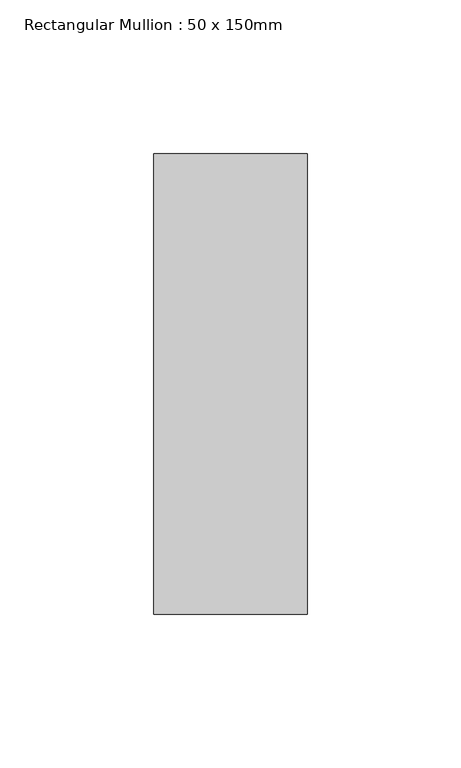
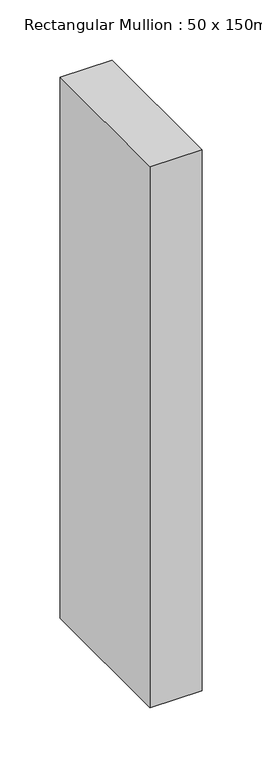
"""IFC4 building model written with IfcOpenShell, lengths in millimetres: member geometry, Rectangular Mullion : 50 x 150mm."""

from ifc_helpers import new_model, si_unit, frame, origin, place, context, project, spatial, polyline, outline, extrude, source, transform, mapped, element, save


def rectangular_mullion_50_x_150mm_b8dbbb25(model_context):
    return source(origin(), model_context, "Body", "SweptSolid", [
        extrude(outline(polyline([(25.0, 75.0), (25.0, -75.0), (-25.0, -75.0), (-25.0, 75.0), (25.0, 75.0)])), frame((0.0, 0.0, -550.0), z_axis=(0.0, 0.0, 1.0), x_axis=(1.0, 0.0, 0.0)), (0.0, 0.0, 1.0), 550.0),
    ])


if __name__ == "__main__":
    model = new_model("IFC4")
    model_context = context("Model", 3, world=origin())
    ifc_project = project(units=[si_unit("LENGTHUNIT", "METRE", prefix="MILLI")], contexts=[model_context])
    site = spatial("IfcSite", under=ifc_project)
    building = spatial("IfcBuilding", under=site)
    placement = place(None, origin())
    rectangular_mullion_50_x_150mm_shape = rectangular_mullion_50_x_150mm_b8dbbb25(model_context)
    element("IfcMember", 1, ObjectType="Rectangular Mullion : 50 x 150mm", at=placement, inside=building, context=model_context, shape_type="MappedRepresentation", body=[
        mapped(rectangular_mullion_50_x_150mm_shape, transform((0.0, 0.0, 0.0), x_axis=(1.0, 0.0, 0.0), y_axis=(0.0, 1.0, 0.0), z_axis=(0.0, 0.0, 1.0))),
    ])
    save(model, "model.ifc")

# Revit data of these elements
# Type "Rectangular Mullion : 50 x 150mm"
#   built-in parameter 1007304 = 0.492126 (stored number, unit not read)
#   built-in parameter 1007301 = 0.082021 (stored number, unit not read)
#   built-in parameter 1007300 = 0.082021 (stored number, unit not read)
# Element 1 (IfcMember, "Rectangular Mullion : 50 x 150mm")
#   Materials on its faces: "Aluminium"
# Materials
#   "Aluminium": class "Metal", colour RGB 247 247 247, transparency 0, Description = "Aluminium 6061", Cost = 0
